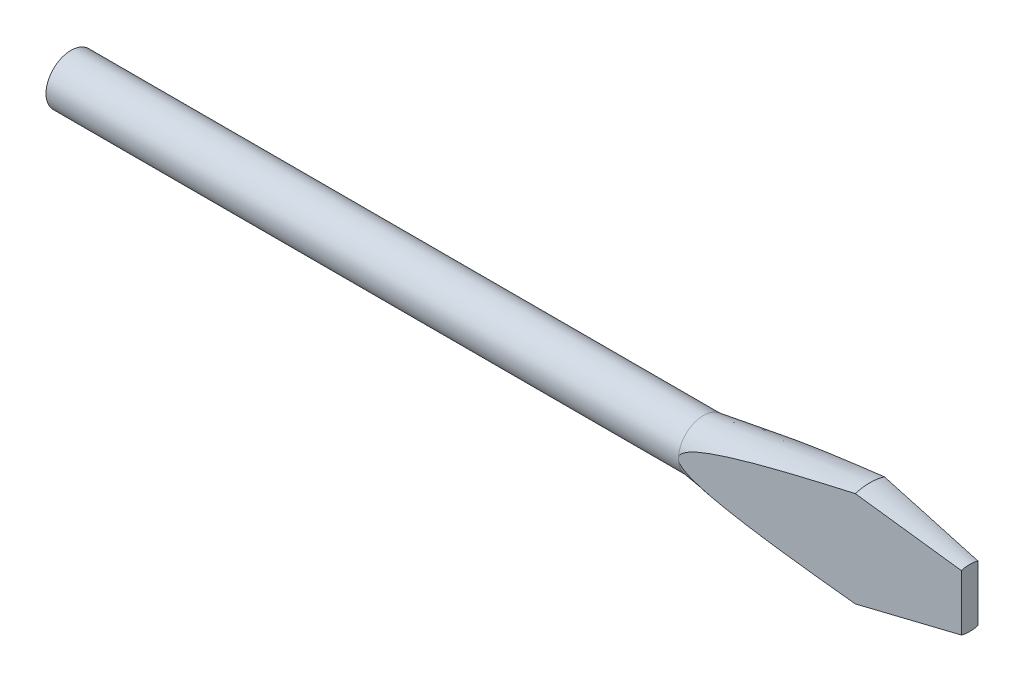
SolidWorks part; units mm, degrees
material "Plain Carbon Steel"
ref_plane "Front Plane" through (0, 0, 0) normal (0, 0, 1) x (1, 0, 0)
ref_plane "Top Plane" through (0, 0, 0) normal (0, 1, 0) x (1, 0, 0)
ref_plane "Right Plane" through (0, 0, 0) normal (1, 0, 0) x (0, 0, -1)
sketch "Shaft Profile Sketch" plane through (0, 0, 0) normal (0, 0, 1) x (1, 0, 0)
  line L0 (-206.405, 0) -> (10113.8449, 0) construction
  line L1 (0, -206.405) -> (0, 10113.8449) construction
  line L2 (0, 0) -> (0, 3)
  line L3 (0, 3) -> (76, 3)
  line L4 (76, 3) -> (96, 6)
  line L5 (96, 6) -> (108, 3.5)
  line L6 (108, 3.5) -> (108, 0)
  line L7 (108, 0) -> (0, 0)
  dimension "D1" = 3.5
  dimension "D2" = 3
  dimension "D3" = 32
  dimension "D4" = 12
  dimension "D5" = 6
  dimension "D6" = 108
revolve "Shaft Revolve" add sketch "Shaft Profile Sketch" angle 360 about L0
sketch "Blade Flat Sketch" plane through (0, 0, 0) normal (0, 1, 0) x (1, 0, 0)
  line L0 (108, 1) -> (76, 3)
  line L1 (108, -3.5) -> (108, 3.5) construction
  line L2 (76, 3) -> (76, 10.728)
  line L3 (76, 10.728) -> (108, 10.728)
  line L4 (108, 10.728) -> (108, 1)
  line L5 (-1000, 0) -> (49000, 0) construction
  dimension "D1" = 1
  dimension "D2" = 7.728
extrude "Blade Flat Cut" cut sketch "Blade Flat Sketch" against normal mid plane 20
mirror "Blade Flat Mirror" about plane through (0, 0, 0) normal (0, 0, 1) of "Blade Flat Cut"
